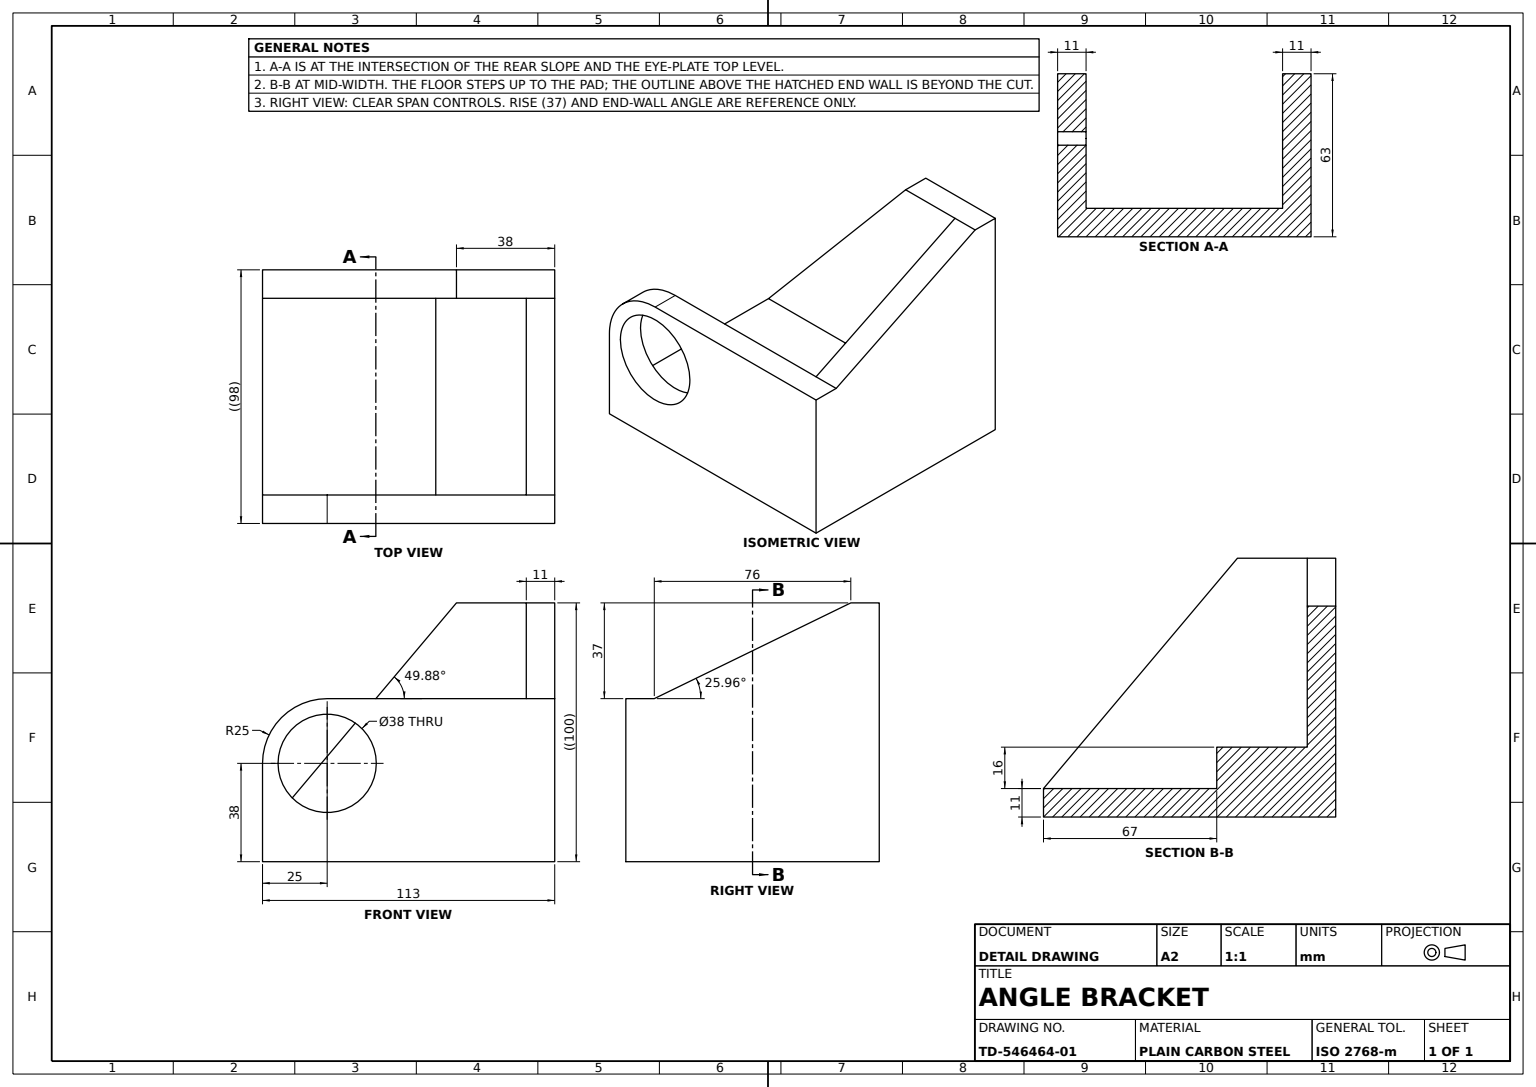
SolidWorks part; units mm, degrees
material "Plain Carbon Steel"
ref_plane "Front Plane" through (0, 0, 0) normal (0, 0, 1) x (1, 0, 0)
ref_plane "Top Plane" through (0, 0, 0) normal (0, 1, 0) x (1, 0, 0)
ref_plane "Right Plane" through (0, 0, 0) normal (1, 0, 0) x (0, 0, -1)
sketch "Eye Plate Profile" plane through (0, 0, 0) normal (0, 0, 1) x (1, 0, 0)
  line L0 (0, 0) -> (113, 0)
  line L1 (113, 0) -> (113, 63)
  line L2 (113, 63) -> (25, 63)
  line L4 (0, 0) -> (0, 38)
  arc A0 (25, 63) -> (0, 38) centre (25, 38) ccw
  dimension "D1" = 50
  dimension "D2" = 25
  dimension "D3" = 113
  dimension "D4" = 63
extrude "Eye Plate 11mm" add sketch "Eye Plate Profile" along normal blind 11
sketch "Floor Plate Profile" plane through (113, 0, 0) normal (1, 0, 0) x (0, 0, -1)
  line L0 (0, 0) -> (76, 0)
  line L1 (76, 0) -> (76, 100)
  line L2 (76, 100) -> (0, 63)
  line L3 (0, 63) -> (0, 0)
  line L4 (0, 0) -> (0, 63) construction
  line L5 (-11, 63) -> (0, 63) construction
  dimension "D1" = 76
  dimension "D2" = 37
extrude "Floor Plate 11mm" add sketch "Floor Plate Profile" against normal blind 11
sketch "Side Wall Profile" plane through (0, 0, -76) normal (0, 0, -1) x (-1, 0, 0)
  line L0 (-113, 0) -> (0, 0)
  line L1 (0, 0) -> (0, 11)
  line L2 (0, 38) -> (0, 0) construction
  line L3 (-113, 0) -> (-113, 100)
  line L4 (-113, 100) -> (-75, 100)
  line L5 (-75, 100) -> (0, 11)
  line L6 (-113, 0) -> (-113, 100) construction
  line L7 (-102, 0) -> (-113, 0) construction
  dimension "D1" = 38
  dimension "D2" = 11
extrude "Side Wall 11mm" add sketch "Side Wall Profile" along normal blind 11
sketch "Inclined Web Profile" plane through (0, 0, 0) normal (0, -1, 0) x (1, 0, 0)
  line L0 (0, 0) -> (102, 0)
  line L1 (102, 0) -> (102, -76)
  line L2 (102, -76) -> (0, -76)
  line L3 (0, -76) -> (0, 0)
extrude "Inclined Web 11mm" add sketch "Inclined Web Profile" against normal blind 11
sketch "End Cap Profile" plane through (0, 11, 0) normal (0, 1, 0) x (1, 0, 0)
  line L0 (0, 0) -> (0, 76) construction
  line L1 (0, 76) -> (102, 76) construction
  line L2 (67, 76) -> (102, 76)
  line L3 (102, 76) -> (102, 0)
  line L4 (102, 0) -> (67, 0)
  line L5 (102, 0) -> (0, 0) construction
  line L6 (67, 0) -> (67, 76)
  dimension "D1" = 67
extrude "End Cap 16mm" add sketch "End Cap Profile" along normal blind 16
sketch "Pivot Bore Profile" plane through (0, 0, 11) normal (0, 0, 1) x (1, 0, 0)
  circle A0 centre (25, 38) radius 19
  dimension "D1" = 38
  dimension "D2" = 38
extrude "Pivot Bore Ø38" cut sketch "Pivot Bore Profile" against normal blind 11
